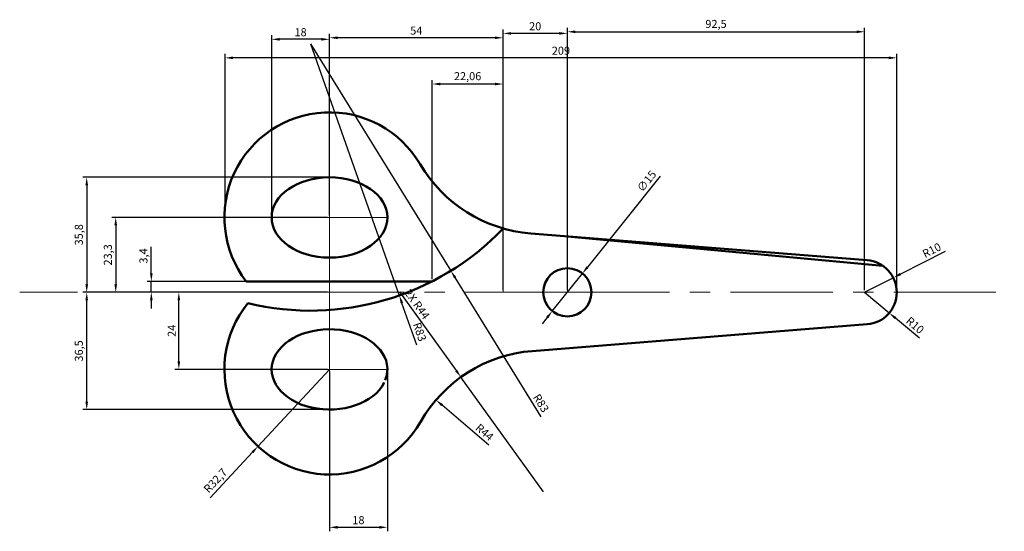
# Model space of a CAD drawing. Units: millimetres. Extents: x 183835 to 184142, y 110902 to 111061.
import ezdxf

# ---------------------------------------------------------------- set-up
doc = ezdxf.new("R2010")
doc.units = ezdxf.units.MM
doc.linetypes.add('CENTER', pattern=[50.8, 31.75, -6.35, 6.35, -6.35])
for name, color, linetype, lineweight in [('M-CNTR', 4, 'CENTER', 18), ('M-CONS', 8, 'Continuous', 13), ('M-DIMS', 2, 'Continuous', 25), ('M-OUTL', 7, 'Continuous', 50)]:
    doc.layers.add(name, color=color, linetype=linetype, lineweight=lineweight)
doc.styles.get("Standard").update_dxf_attribs({"font": 'arial.ttf'})
doc.dimstyles.new('ISO-25', dxfattribs={"dimtxt": 2.5, "dimasz": 2.5, "dimexe": 1.25, "dimexo": 0.625, "dimtad": 1, "dimtxsty": 'Standard', "dimcen": 2.5, "dimadec": 0, "dimazin": 0, "dimtfac": 1, "dimtmove": 0, "dimatfit": 3, "dimfxl": 1, "dimarcsym": 0})

# ---------------------------------------------------------------- blocks, each defined once
blk = doc.blocks.new('*D1')
at = {"layer": 'Defpoints', "color": 0, "transparency": 16777216}
for p in [(184098.32, 111057.44), (184005.82, 110976.37), (184098.32, 110976.37)]:
    blk.add_point(p, dxfattribs=at)
at = {"layer": 'M-DIMS', "color": 0, "lineweight": -2, "transparency": 16777216}
for p, q in [((184005.82, 110977), (184005.82, 111058.69)), ((184008.32, 111057.44), (184095.82, 111057.44)), ((184098.32, 110977), (184098.32, 111058.69))]:
    blk.add_line(p, q, dxfattribs=at)
at = {"layer": 'M-DIMS', "color": 0, "transparency": 16777216}
for points in [[(184008.32, 111057.85), (184008.32, 111057.02), (184005.82, 111057.44)], [(184095.82, 111057.85), (184095.82, 111057.02), (184098.32, 111057.44)]]:
    blk.add_solid(points, dxfattribs=at)
at = {"layer": 'M-DIMS', "color": 0, "transparency": 16777216, "insert": (184052.07, 111059.56), "char_height": 2.5, "attachment_point": 5}
blk.add_mtext('92,5', dxfattribs=at)
blk = doc.blocks.new('*D2')
at = {"layer": 'Defpoints', "color": 0, "transparency": 16777216}
for p in [(183985.82, 111056.93), (183985.82, 110976.37), (184005.82, 110976.37)]:
    blk.add_point(p, dxfattribs=at)
at = {"layer": 'M-DIMS', "color": 0, "lineweight": -2, "transparency": 16777216}
for p, q in [((183985.82, 110977), (183985.82, 111058.18)), ((184005.82, 110977), (184005.82, 111058.18)), ((184003.32, 111056.93), (183988.32, 111056.93))]:
    blk.add_line(p, q, dxfattribs=at)
at = {"layer": 'M-DIMS', "color": 0, "transparency": 16777216}
for points in [[(183988.32, 111057.35), (183988.32, 111056.52), (183985.82, 111056.93)], [(184003.32, 111057.35), (184003.32, 111056.52), (184005.82, 111056.93)]]:
    blk.add_solid(points, dxfattribs=at)
at = {"layer": 'M-DIMS', "color": 0, "transparency": 16777216, "insert": (183995.82, 111058.84), "char_height": 2.5, "attachment_point": 5}
blk.add_mtext('20', dxfattribs=at)
blk = doc.blocks.new('*D3')
at = {"layer": 'Defpoints', "color": 0, "transparency": 16777216}
for p in [(183931.82, 111055.58), (183931.82, 110999.67), (183985.82, 110976.37)]:
    blk.add_point(p, dxfattribs=at)
at = {"layer": 'M-DIMS', "color": 0, "lineweight": -2, "transparency": 16777216}
for p, q in [((183931.82, 111000.3), (183931.82, 111056.83)), ((183983.32, 111055.58), (183934.32, 111055.58)), ((183985.82, 110977), (183985.82, 111056.83))]:
    blk.add_line(p, q, dxfattribs=at)
at = {"layer": 'M-DIMS', "color": 0, "transparency": 16777216}
for points in [[(183934.32, 111055.99), (183934.32, 111055.16), (183931.82, 111055.58)], [(183983.32, 111055.99), (183983.32, 111055.16), (183985.82, 111055.58)]]:
    blk.add_solid(points, dxfattribs=at)
at = {"layer": 'M-DIMS', "color": 0, "transparency": 16777216, "insert": (183958.82, 111057.47), "char_height": 2.5, "attachment_point": 5}
blk.add_mtext('54', dxfattribs=at)
blk = doc.blocks.new('*D4')
at = {"layer": 'Defpoints', "color": 0, "transparency": 16777216}
for p in [(183963.76, 111041.18), (183963.76, 110979.77), (183985.82, 110976.37)]:
    blk.add_point(p, dxfattribs=at)
at = {"layer": 'M-DIMS', "color": 0, "lineweight": -2, "transparency": 16777216}
for p, q in [((183963.76, 110980.4), (183963.76, 111042.43)), ((183985.82, 110977), (183985.82, 111042.43)), ((183983.32, 111041.18), (183966.26, 111041.18))]:
    blk.add_line(p, q, dxfattribs=at)
at = {"layer": 'M-DIMS', "color": 0, "transparency": 16777216}
for points in [[(183966.26, 111041.59), (183966.26, 111040.76), (183963.76, 111041.18)], [(183983.32, 111041.59), (183983.32, 111040.76), (183985.82, 111041.18)]]:
    blk.add_solid(points, dxfattribs=at)
at = {"layer": 'M-DIMS', "color": 0, "transparency": 16777216, "insert": (183974.79, 111043.31), "char_height": 2.5, "attachment_point": 5}
blk.add_mtext('22,06', dxfattribs=at)
blk = doc.blocks.new('*D5')
at = {"layer": 'Defpoints', "color": 0, "transparency": 16777216}
for p in [(183913.82, 111055.09), (183913.82, 110999.67), (183931.82, 110999.67)]:
    blk.add_point(p, dxfattribs=at)
at = {"layer": 'M-DIMS', "color": 0, "lineweight": -2, "transparency": 16777216}
for p, q in [((183913.82, 111000.3), (183913.82, 111056.34)), ((183929.32, 111055.09), (183916.32, 111055.09)), ((183931.82, 111000.3), (183931.82, 111056.34))]:
    blk.add_line(p, q, dxfattribs=at)
at = {"layer": 'M-DIMS', "color": 0, "transparency": 16777216}
for points in [[(183916.32, 111055.51), (183916.32, 111054.68), (183913.82, 111055.09)], [(183929.32, 111055.51), (183929.32, 111054.68), (183931.82, 111055.09)]]:
    blk.add_solid(points, dxfattribs=at)
at = {"layer": 'M-DIMS', "color": 0, "transparency": 16777216, "insert": (183922.82, 111056.99), "char_height": 2.5, "attachment_point": 5}
blk.add_mtext('18', dxfattribs=at)
blk = doc.blocks.new('*D6')
at = {"layer": 'Defpoints', "color": 0, "transparency": 16777216}
for p in [(183931.82, 110952.37), (183949.82, 110952.37), (183949.82, 110903.23)]:
    blk.add_point(p, dxfattribs=at)
at = {"layer": 'M-DIMS', "color": 0, "lineweight": -2, "transparency": 16777216}
for p, q in [((183931.82, 110951.75), (183931.82, 110901.98)), ((183949.82, 110951.75), (183949.82, 110901.98)), ((183934.32, 110903.23), (183947.32, 110903.23))]:
    blk.add_line(p, q, dxfattribs=at)
at = {"layer": 'M-DIMS', "color": 0, "transparency": 16777216}
for points in [[(183934.32, 110903.65), (183934.32, 110902.81), (183931.82, 110903.23)], [(183947.32, 110903.65), (183947.32, 110902.81), (183949.82, 110903.23)]]:
    blk.add_solid(points, dxfattribs=at)
at = {"layer": 'M-DIMS', "color": 0, "transparency": 16777216, "insert": (183940.82, 110905.13), "char_height": 2.5, "attachment_point": 5}
blk.add_mtext('18', dxfattribs=at)
blk = doc.blocks.new('*D7')
at = {"layer": 'Defpoints', "color": 0, "transparency": 16777216}
for p in [(183884.94, 110976.37), (183931.82, 110976.37), (183931.82, 110952.37)]:
    blk.add_point(p, dxfattribs=at)
at = {"layer": 'M-DIMS', "color": 0, "lineweight": -2, "transparency": 16777216}
for p, q in [((183931.2, 110976.37), (183883.69, 110976.37)), ((183884.94, 110954.87), (183884.94, 110973.87)), ((183931.2, 110952.37), (183883.69, 110952.37))]:
    blk.add_line(p, q, dxfattribs=at)
at = {"layer": 'M-DIMS', "color": 0, "transparency": 16777216}
for points in [[(183884.52, 110973.87), (183885.35, 110973.87), (183884.94, 110976.37)], [(183884.52, 110954.87), (183885.35, 110954.87), (183884.94, 110952.37)]]:
    blk.add_solid(points, dxfattribs=at)
at = {"layer": 'M-DIMS', "color": 0, "transparency": 16777216, "insert": (183883.06, 110964.37), "char_height": 2.5, "attachment_point": 5, "rotation": 90}
blk.add_mtext('24', dxfattribs=at)
blk = doc.blocks.new('*D8')
at = {"layer": 'Defpoints', "color": 0, "transparency": 16777216}
for p in [(183876.37, 110979.77), (183907.44, 110979.77), (183907.44, 110976.37)]:
    blk.add_point(p, dxfattribs=at)
at = {"layer": 'M-DIMS', "color": 0, "lineweight": -2, "transparency": 16777216}
for p, q in [((183876.37, 110982.27), (183876.37, 110990.56)), ((183906.82, 110979.77), (183875.12, 110979.77)), ((183876.37, 110976.37), (183876.37, 110979.77)), ((183906.82, 110976.37), (183875.12, 110976.37)), ((183876.37, 110973.87), (183876.37, 110971.37))]:
    blk.add_line(p, q, dxfattribs=at)
at = {"layer": 'M-DIMS', "color": 0, "transparency": 16777216}
for points in [[(183875.96, 110982.27), (183876.79, 110982.27), (183876.37, 110979.77)], [(183875.96, 110973.87), (183876.79, 110973.87), (183876.37, 110976.37)]]:
    blk.add_solid(points, dxfattribs=at)
at = {"layer": 'M-DIMS', "color": 0, "transparency": 16777216, "insert": (183874.25, 110987.66), "char_height": 2.5, "attachment_point": 5, "rotation": 90}
blk.add_mtext('3,4', dxfattribs=at)
blk = doc.blocks.new('*D9')
at = {"layer": 'Defpoints', "color": 0, "transparency": 16777216}
for p in [(183931.82, 110999.67), (183865.3, 110976.37), (183931.82, 110976.37)]:
    blk.add_point(p, dxfattribs=at)
at = {"layer": 'M-DIMS', "color": 0, "lineweight": -2, "transparency": 16777216}
for p, q in [((183931.2, 110999.67), (183864.05, 110999.67)), ((183865.3, 110997.17), (183865.3, 110978.87)), ((183931.2, 110976.37), (183864.05, 110976.37))]:
    blk.add_line(p, q, dxfattribs=at)
at = {"layer": 'M-DIMS', "color": 0, "transparency": 16777216}
for points in [[(183864.88, 110997.17), (183865.71, 110997.17), (183865.3, 110999.67)], [(183864.88, 110978.87), (183865.71, 110978.87), (183865.3, 110976.37)]]:
    blk.add_solid(points, dxfattribs=at)
at = {"layer": 'M-DIMS', "color": 0, "transparency": 16777216, "insert": (183863.17, 110988.02), "char_height": 2.5, "attachment_point": 5, "rotation": 90}
blk.add_mtext('23,3', dxfattribs=at)
blk = doc.blocks.new('*D10')
at = {"layer": 'Defpoints', "color": 0, "transparency": 16777216}
for p in [(183931.82, 111012.17), (183856.28, 110976.37), (183931.82, 110976.37)]:
    blk.add_point(p, dxfattribs=at)
at = {"layer": 'M-DIMS', "color": 0, "lineweight": -2, "transparency": 16777216}
for p, q in [((183931.2, 111012.17), (183855.03, 111012.17)), ((183856.28, 111009.67), (183856.28, 110978.87)), ((183931.2, 110976.37), (183855.03, 110976.37))]:
    blk.add_line(p, q, dxfattribs=at)
at = {"layer": 'M-DIMS', "color": 0, "transparency": 16777216}
for points in [[(183855.86, 111009.67), (183856.69, 111009.67), (183856.28, 111012.17)], [(183855.86, 110978.87), (183856.69, 110978.87), (183856.28, 110976.37)]]:
    blk.add_solid(points, dxfattribs=at)
at = {"layer": 'M-DIMS', "color": 0, "transparency": 16777216, "insert": (183854.15, 110994.27), "char_height": 2.5, "attachment_point": 5, "rotation": 90}
blk.add_mtext('35,8', dxfattribs=at)
blk = doc.blocks.new('*D11')
at = {"layer": 'Defpoints', "color": 0, "transparency": 16777216}
for p in [(183856.28, 110976.37), (183931.2, 110976.37), (183931.82, 110939.87)]:
    blk.add_point(p, dxfattribs=at)
at = {"layer": 'M-DIMS', "color": 0, "lineweight": -2, "transparency": 16777216}
for p, q in [((183930.57, 110976.37), (183855.03, 110976.37)), ((183856.28, 110942.37), (183856.28, 110973.87)), ((183931.2, 110939.87), (183855.03, 110939.87))]:
    blk.add_line(p, q, dxfattribs=at)
at = {"layer": 'M-DIMS', "color": 0, "transparency": 16777216}
for points in [[(183855.86, 110973.87), (183856.69, 110973.87), (183856.28, 110976.37)], [(183855.86, 110942.37), (183856.69, 110942.37), (183856.28, 110939.87)]]:
    blk.add_solid(points, dxfattribs=at)
at = {"layer": 'M-DIMS', "color": 0, "transparency": 16777216, "insert": (183854.15, 110958.12), "char_height": 2.5, "attachment_point": 5, "rotation": 90}
blk.add_mtext('36,5', dxfattribs=at)
blk = doc.blocks.new('*D12')
at = {"layer": 'Defpoints', "color": 0, "transparency": 16777216}
for p in [(184107.24, 110980.9), (184098.32, 110976.37)]:
    blk.add_point(p, dxfattribs=at)
at = {"layer": 'M-DIMS', "color": 0, "lineweight": -2, "transparency": 16777216}
for p, q in [((184123.41, 110989.11), (184109.47, 110982.03)), ((184098.32, 110976.37), (184107.24, 110980.9))]:
    blk.add_line(p, q, dxfattribs=at)
at = {"layer": 'M-DIMS', "color": 0, "transparency": 16777216}
blk.add_solid([(184109.28, 110982.4), (184109.66, 110981.66), (184107.24, 110980.9)], dxfattribs=at)
at = {"layer": 'M-DIMS', "color": 0, "transparency": 16777216, "insert": (184119.33, 110989.17), "char_height": 2.5, "attachment_point": 5, "rotation": 26.9163}
blk.add_mtext('R10', dxfattribs=at)
blk = doc.blocks.new('*D13')
at = {"layer": 'Defpoints', "color": 0, "transparency": 16777216}
for p in [(184010.5, 110982.23), (184001.14, 110970.51)]:
    blk.add_point(p, dxfattribs=at)
at = {"layer": 'M-DIMS', "color": 0, "lineweight": -2, "transparency": 16777216}
for p, q in [((184034.65, 111012.48), (184012.06, 110984.19)), ((184001.14, 110970.51), (184010.5, 110982.23)), ((183999.58, 110968.56), (183998.02, 110966.6))]:
    blk.add_line(p, q, dxfattribs=at)
at = {"layer": 'M-DIMS', "color": 0, "transparency": 16777216}
for points in [[(184011.74, 110984.45), (184012.39, 110983.93), (184010.5, 110982.23)], [(183999.26, 110968.82), (183999.91, 110968.3), (184001.14, 110970.51)]]:
    blk.add_solid(points, dxfattribs=at)
at = {"layer": 'M-DIMS', "color": 0, "transparency": 16777216, "insert": (184030.74, 111010.75), "char_height": 2.5, "attachment_point": 5, "rotation": 51.3978}
blk.add_mtext('∅15', dxfattribs=at)
blk = doc.blocks.new('*D14')
at = {"layer": 'Defpoints', "color": 0, "transparency": 16777216}
for p in [(183931.82, 110952.37), (183909.56, 110928.42)]:
    blk.add_point(p, dxfattribs=at)
at = {"layer": 'M-DIMS', "color": 0, "lineweight": -2, "transparency": 16777216}
for p, q in [((183931.82, 110952.37), (183909.56, 110928.42)), ((183894.66, 110912.39), (183907.86, 110926.59))]:
    blk.add_line(p, q, dxfattribs=at)
at = {"layer": 'M-DIMS', "color": 0, "transparency": 16777216}
blk.add_solid([(183907.55, 110926.87), (183908.16, 110926.31), (183909.56, 110928.42)], dxfattribs=at)
at = {"layer": 'M-DIMS', "color": 0, "transparency": 16777216, "insert": (183896.55, 110917.55), "char_height": 2.5, "attachment_point": 5, "rotation": 47.0878}
blk.add_mtext('R32,7', dxfattribs=at)
blk = doc.blocks.new('*D15')
at = {"layer": 'Defpoints', "color": 0, "transparency": 16777216}
for p in [(183925.93, 111053.65), (183953.52, 110975.37)]:
    blk.add_point(p, dxfattribs=at)
at = {"layer": 'M-DIMS', "color": 0, "lineweight": -2, "transparency": 16777216}
for p, q in [((183925.93, 111053.65), (183953.52, 110975.37)), ((183958.98, 110959.9), (183954.36, 110973.01))]:
    blk.add_line(p, q, dxfattribs=at)
at = {"layer": 'M-DIMS', "color": 0, "transparency": 16777216}
blk.add_solid([(183954.75, 110973.15), (183953.96, 110972.87), (183953.52, 110975.37)], dxfattribs=at)
at = {"layer": 'M-DIMS', "color": 0, "transparency": 16777216, "insert": (183959.57, 110963.94), "char_height": 2.5, "attachment_point": 5, "rotation": 289.4181}
blk.add_mtext('R83', dxfattribs=at)
blk = doc.blocks.new('*D16')
at = {"layer": 'Defpoints', "color": 0, "transparency": 16777216}
for p in [(183964.95, 110942.86), (183998.37, 110914.23)]:
    blk.add_point(p, dxfattribs=at)
at = {"layer": 'M-DIMS', "color": 0, "lineweight": -2, "transparency": 16777216}
blk.add_line((183981.37, 110928.79), (183966.85, 110941.23), dxfattribs=at)
at = {"layer": 'M-DIMS', "color": 0, "transparency": 16777216}
blk.add_solid([(183967.12, 110941.55), (183966.58, 110940.91), (183964.95, 110942.86)], dxfattribs=at)
at = {"layer": 'M-DIMS', "color": 0, "transparency": 16777216, "insert": (183979.85, 110932.56), "char_height": 2.5, "attachment_point": 5, "rotation": 319.4153}
blk.add_mtext('R44', dxfattribs=at)
blk = doc.blocks.new('*D17')
at = {"layer": 'Defpoints', "color": 0, "transparency": 16777216}
for p in [(183899.32, 111049.33), (183899.32, 110996.07), (184108.32, 110976.37)]:
    blk.add_point(p, dxfattribs=at)
at = {"layer": 'M-DIMS', "color": 0, "lineweight": -2, "transparency": 16777216}
for p, q in [((183899.32, 110996.7), (183899.32, 111050.58)), ((184105.82, 111049.33), (183901.82, 111049.33)), ((184108.32, 110977), (184108.32, 111050.58))]:
    blk.add_line(p, q, dxfattribs=at)
at = {"layer": 'M-DIMS', "color": 0, "transparency": 16777216}
for points in [[(183901.82, 111049.75), (183901.82, 111048.91), (183899.32, 111049.33)], [(184105.82, 111049.75), (184105.82, 111048.91), (184108.32, 111049.33)]]:
    blk.add_solid(points, dxfattribs=at)
at = {"layer": 'M-DIMS', "color": 0, "transparency": 16777216, "insert": (184003.82, 111051.23), "char_height": 2.5, "attachment_point": 5}
blk.add_mtext('209', dxfattribs=at)
blk = doc.blocks.new('*D18')
at = {"layer": 'Defpoints', "color": 0, "transparency": 16777216}
for p in [(184098.32, 110976.37), (184105.98, 110969.94)]:
    blk.add_point(p, dxfattribs=at)
at = {"layer": 'M-DIMS', "color": 0, "lineweight": -2, "transparency": 16777216}
for p, q in [((184098.32, 110976.37), (184105.98, 110969.94)), ((184115.34, 110962.08), (184107.89, 110968.33))]:
    blk.add_line(p, q, dxfattribs=at)
at = {"layer": 'M-DIMS', "color": 0, "transparency": 16777216}
blk.add_solid([(184108.16, 110968.65), (184107.63, 110968.01), (184105.98, 110969.94)], dxfattribs=at)
at = {"layer": 'M-DIMS', "color": 0, "transparency": 16777216, "insert": (184113.79, 110965.86), "char_height": 2.5, "attachment_point": 5, "rotation": 319.9801}
blk.add_mtext('R10', dxfattribs=at)
blk = doc.blocks.new('*D19')
at = {"layer": 'Defpoints', "color": 0, "transparency": 16777216}
for p in [(183972.69, 110949.96), (183998.37, 110914.23)]:
    blk.add_point(p, dxfattribs=at)
at = {"layer": 'M-DIMS', "color": 0, "lineweight": -2, "transparency": 16777216}
for p, q in [((183953.59, 110976.52), (183971.23, 110951.99)), ((183998.37, 110914.23), (183972.69, 110949.96))]:
    blk.add_line(p, q, dxfattribs=at)
at = {"layer": 'M-DIMS', "color": 0, "transparency": 16777216}
blk.add_solid([(183971.57, 110952.23), (183970.89, 110951.75), (183972.69, 110949.96)], dxfattribs=at)
at = {"layer": 'M-DIMS', "color": 0, "transparency": 16777216, "insert": (183958.8, 110972.49), "char_height": 2.5, "attachment_point": 5, "rotation": 305.7088}
blk.add_mtext('2X R44', dxfattribs=at)
blk = doc.blocks.new('*D20')
at = {"layer": 'Defpoints', "color": 0, "transparency": 16777216}
for p in [(183925.93, 111053.65), (183969.57, 110983.05)]:
    blk.add_point(p, dxfattribs=at)
at = {"layer": 'M-DIMS', "color": 0, "lineweight": -2, "transparency": 16777216}
for p, q in [((183925.93, 111053.65), (183969.57, 110983.05)), ((183997.66, 110937.61), (183970.89, 110980.92))]:
    blk.add_line(p, q, dxfattribs=at)
at = {"layer": 'M-DIMS', "color": 0, "transparency": 16777216}
blk.add_solid([(183971.24, 110981.14), (183970.53, 110980.7), (183969.57, 110983.05)], dxfattribs=at)
at = {"layer": 'M-DIMS', "color": 0, "transparency": 16777216, "insert": (183997.37, 110941.69), "char_height": 2.5, "attachment_point": 5, "rotation": 301.7222}
blk.add_mtext('R83', dxfattribs=at)

msp = doc.modelspace()

# ---------------------------------------------------------------- linework, layer by layer
at = {"layer": 'M-CNTR'}
for p, q in [((183931.822, 110976.37), (183931.822, 111012.17)), ((183931.822, 110999.67), (183913.822, 110999.67)), ((183931.822, 110976.37), (183931.822, 110999.67)), ((183931.822, 110999.67), (183949.822, 110999.67)), ((184005.822, 110976.37), (183835.42, 110976.37)), ((183931.822, 110976.37), (183931.822, 110952.37)), ((183931.822, 110976.37), (183931.822, 110939.87)), ((184005.822, 110976.37), (184141.776, 110976.37)), ((183931.822, 110952.37), (183931.822, 110964.87)), ((183931.822, 110952.37), (183913.822, 110952.37)), ((183931.822, 110952.37), (183949.427, 110952.37)), ((183931.822, 110952.37), (183949.822, 110952.37))]:
    msp.add_line(p, q, dxfattribs=at)
at = {"layer": 'M-CONS'}
for p, q in [((183985.822, 110995.37), (183985.822, 110996.246)), ((183985.822, 110976.37), (183985.822, 110995.37)), ((183985.822, 110976.37), (183985.822, 110995.37)), ((184005.822, 110976.37), (184005.822, 110993.776)), ((183931.822, 110976.37), (183931.822, 110979.77)), ((183931.822, 110976.37), (183931.822, 110972.97)), ((183931.822, 110976.37), (183931.822, 110972.97))]:
    msp.add_line(p, q, dxfattribs=at)
at = {"layer": 'M-OUTL'}
for p, q in [((183994.445, 110994.683), (184099.117, 110986.339)), ((184103.974, 110984.62), (184005.822, 110993.776)), ((183931.822, 110979.77), (183905.875, 110979.77)), ((183931.822, 110979.77), (183960.888, 110979.77)), ((183960.888, 110979.77), (183963.763, 110979.77)), ((183994.871, 110958.092), (184099.117, 110966.402))]:
    msp.add_line(p, q, dxfattribs=at)
msp.add_circle((184005.822, 110976.37), 7.5, dxfattribs=at)
for centre, radius, start, end in [((183931.822, 110999.67), 32.7, 30.45257, 217.48565), ((183997.941, 111038.544), 44, 210.45257, 265.44213), ((183925.93, 111053.646), 83, 256.40945, 316.18593), ((184098.322, 110976.37), 10, 274.55787, 85.44213), ((183931.822, 110952.37), 32.7, 140.95213, 330.1814), ((183998.367, 110914.231), 44, 94.55787, 150.1814)]:
    msp.add_arc(centre, radius, start, end, dxfattribs=at)
msp.add_ellipse((183931.822, 110999.67), major_axis=(18, 0), ratio=0.6944444, dxfattribs=at)
msp.add_ellipse((183931.822, 110952.37), major_axis=(18, 0), ratio=0.6944444, start_param=6.0103351, end_param=12.237424, dxfattribs=at)

# ---------------------------------------------------------------- dimensions: what is measured, and where the dimension line sits
at = {"layer": 'M-DIMS'}
for base, p1, p2, override, picture, middle in [((183985.822, 111056.934), (184005.822, 110976.37), (183985.822, 110976.37), {"dimclrd": 0, "dimclre": 0, "dimclrt": 0}, '*D2', (183995.822, 111058.835)), ((184098.322, 111057.436), (184005.822, 110976.37), (184098.322, 110976.37), {"dimclrd": 0, "dimclre": 0, "dimclrt": 0}, '*D1', (184052.072, 111059.563)), ((183913.822, 111055.093), (183931.822, 110999.67), (183913.822, 110999.67), {"dimclrd": 0, "dimclre": 0, "dimclrt": 0}, '*D5', (183922.822, 111056.995)), ((183931.822, 111055.577), (183985.822, 110976.37), (183931.822, 110999.67), {"dimclrd": 0, "dimclre": 0, "dimclrt": 0}, '*D3', (183958.822, 111057.473)), ((183899.32, 111049.331), (184108.322, 110976.37), (183899.32, 110996.074), {"dimdec": 0, "dimlfac": 1, "dimrnd": 0, "dimzin": 0, "dimdsep": 46, "dimlunit": 2}, '*D17', (184003.821, 111051.233)), ((183963.763, 111041.178), (183985.822, 110976.37), (183963.763, 110979.77), {"dimclrd": 0, "dimclre": 0, "dimclrt": 0}, '*D4', (183974.793, 111043.306)), ((183949.822, 110903.231), (183931.822, 110952.37), (183949.822, 110952.37), {"dimclrd": 0, "dimclre": 0, "dimclrt": 0}, '*D6', (183940.822, 110905.132))]:
    dim = msp.add_linear_dim(base=base, p1=p1, p2=p2, dimstyle='ISO-25', override=override, dxfattribs=at)
    dim.commit()
    dim.dimension.update_dxf_attribs({"geometry": picture, "text_midpoint": middle})
for center, mpoint, override, picture, middle in [((183925.93, 111053.646), (183953.524, 110975.367), {"dimclrd": 0, "dimclre": 0, "dimclrt": 0}, '*D15', (183957.777, 110963.304)), ((183925.93, 111053.646), (183969.572, 110983.046), {"dimdec": 0, "dimlfac": 1, "dimrnd": 0, "dimzin": 0, "dimdsep": 46, "dimlunit": 2}, '*D20', (183995.757, 110940.686)), ((184098.322, 110976.37), (184107.239, 110980.897), {"dimclrd": 0, "dimclre": 0, "dimclrt": 0}, '*D12', (184120.192, 110987.473)), ((183931.822, 110952.37), (183909.557, 110928.421), {"dimclrd": 0, "dimclre": 0, "dimclrt": 0}, '*D14', (183898.109, 110916.106)), ((183998.367, 110914.231), (183964.952, 110942.856), {"dimclrd": 0, "dimclre": 0, "dimclrt": 0}, '*D16', (183978.634, 110931.135))]:
    dim = msp.add_radius_dim(center=center, mpoint=mpoint, dimstyle='ISO-25', override=override, dxfattribs=at)
    dim.commit()
    dim.dimension.update_dxf_attribs({"geometry": picture, "text_midpoint": middle, "dimtype": 164})
dim = msp.add_diameter_dim_2p(p1=(184001.143, 110970.509), p2=(184010.501, 110982.231), dimstyle='ISO-25', override={"dimclrd": 0, "dimclre": 0, "dimclrt": 0}, dxfattribs=at)
dim.commit()
dim.dimension.update_dxf_attribs({"geometry": '*D13', "text_midpoint": (184032.285, 111009.517), "dimtype": 163})
for base, p1, p2, picture, middle in [((183856.276, 110976.37), (183931.822, 111012.17), (183931.822, 110976.37), '*D10', (183854.149, 110994.27)), ((183865.297, 110976.37), (183931.822, 110999.67), (183931.822, 110976.37), '*D9', (183863.169, 110988.02)), ((183876.373, 110979.77), (183907.441, 110976.37), (183907.441, 110979.77), '*D8', (183874.246, 110987.665)), ((183856.276, 110976.37), (183931.822, 110939.87), (183931.197, 110976.37), '*D11', (183854.149, 110958.12)), ((183884.935, 110976.37), (183931.822, 110952.37), (183931.822, 110976.37), '*D7', (183883.055, 110964.37))]:
    dim = msp.add_linear_dim(base=base, p1=p1, p2=p2, angle=90, dimstyle='ISO-25', override={"dimclrd": 0, "dimclre": 0, "dimclrt": 0}, dxfattribs=at)
    dim.commit()
    dim.dimension.update_dxf_attribs({"geometry": picture, "text_midpoint": middle})
dim = msp.add_radius_dim(center=(183998.367, 110914.231), mpoint=(183972.686, 110949.958), text='2X <>', dimstyle='ISO-25', override={"dimdec": 0, "dimlfac": 1, "dimrnd": 0, "dimzin": 0, "dimdsep": 46, "dimlunit": 2}, dxfattribs=at)
dim.commit()
dim.dimension.update_dxf_attribs({"geometry": '*D19', "text_midpoint": (183957.277, 110971.395), "dimtype": 164})
dim = msp.add_radius_dim(center=(184098.322, 110976.37), mpoint=(184105.98, 110969.94), dimstyle='ISO-25', override={"dimdec": 0, "dimlfac": 1, "dimrnd": 0, "dimzin": 0, "dimdsep": 46, "dimlunit": 2}, dxfattribs=at)
dim.commit()
dim.dimension.update_dxf_attribs({"geometry": '*D18', "text_midpoint": (184113.795, 110965.861)})

doc.saveas('drawing.dxf')
